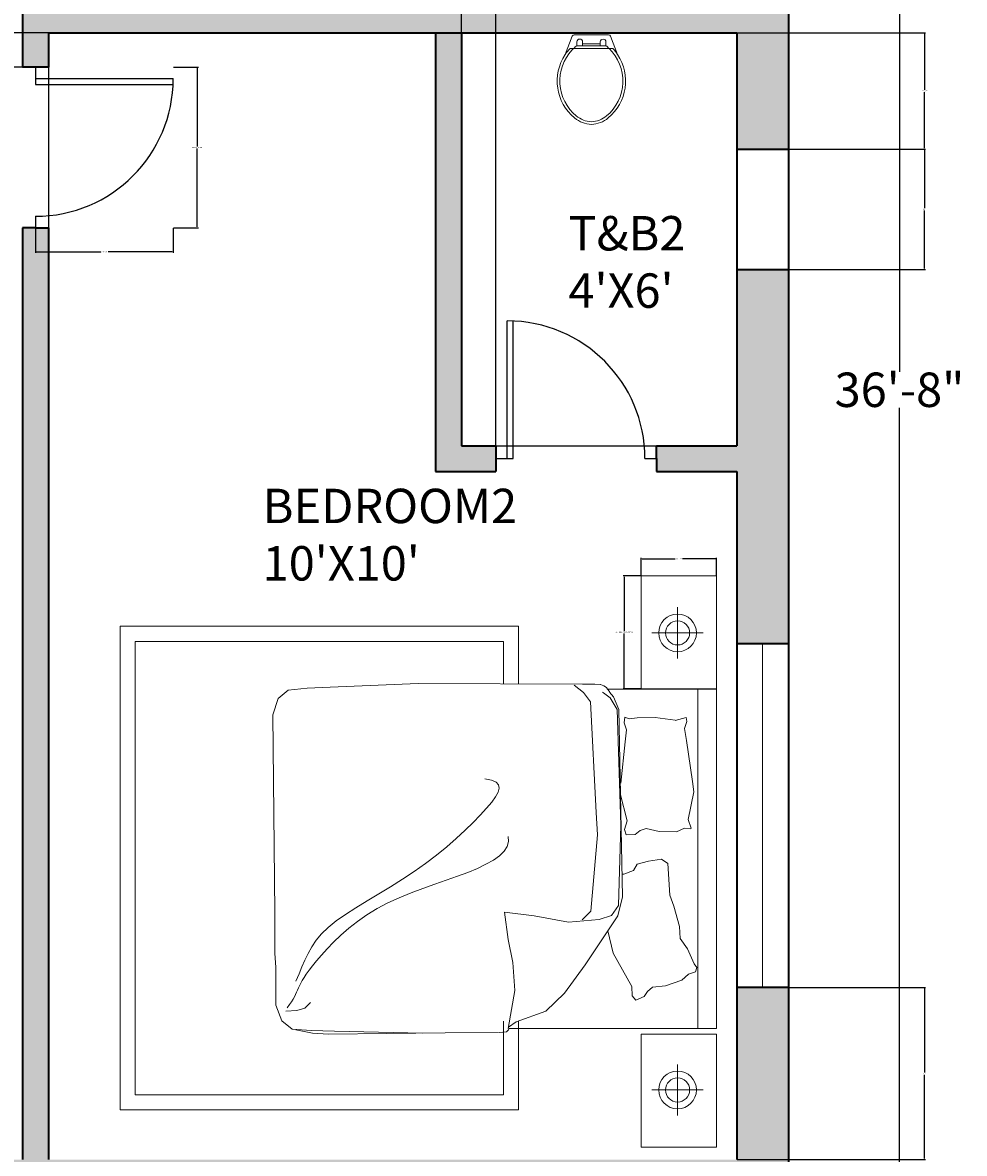
# Model space of a CAD drawing. Units: inches. Extents: x 10 to 332, y -471 to 73.
# Tile 3 of 5: x 168 to 332, y -341 to -144. Entities that reach past the tile are written whole.
import ezdxf

# ---------------------------------------------------------------- set-up
doc = ezdxf.new("R2010")
doc.units = ezdxf.units.IN
doc.header["$MEASUREMENT"] = 0
for name, color, linetype, lineweight in [('A-ANNO-DIMS', 2, 'Continuous', 18), ('A-AREA-IDEN', 7, 'Continuous', 18), ('A-DOOR', 3, 'Continuous', 25), ('A-FURN', 9, 'Continuous', 18), ('A-GLAZ', 4, 'Continuous', 18), ('A-WALL', 7, 'Continuous', 35), ('A-WALL-PATT', 8, 'Continuous', 13), ('WC-Detail_dwgmodels.com', 251, 'Continuous', 13), ('WC-Outline_dwgmodels.com', 250, 'Continuous', 18)]:
    doc.layers.add(name, color=color, linetype=linetype, lineweight=lineweight)
doc.styles.get("Standard").update_dxf_attribs({"font": 'arial.ttf'})
doc.dimstyles.get("Standard").update_dxf_attribs({"dimtxt": 0.18, "dimasz": 0.18, "dimexe": 0.18, "dimexo": 0.0625, "dimgap": 0.09, "dimtad": 0, "dimtih": 1, "dimtoh": 1, "dimdec": 0, "dimzin": 0, "dimdsep": 46, "dimlunit": 3, "dimtxsty": 'Standard', "dimcen": 0.09, "dimadec": 0, "dimazin": 0, "dimtfac": 1, "dimtdec": 0, "dimtofl": 0, "dimtmove": 0, "dimatfit": 3, "dimfxl": 1, "dimtolj": 1, "dimtzin": 0, "dimarcsym": 0})

# ---------------------------------------------------------------- blocks, each defined once
blk = doc.blocks.new('*D3')
at = {"layer": 'A-ANNO-DIMS', "color": 0, "lineweight": -2, "transparency": 16777216}
for p, q in [((301.43, 11.99), (320.92, 11.99)), ((320.74, 11.81), (320.74, -204.61)), ((320.74, -427.33), (320.74, -210.92)), ((301.43, -427.51), (320.92, -427.51))]:
    blk.add_line(p, q, dxfattribs=at)
at = {"layer": 'A-ANNO-DIMS', "color": 0, "transparency": 16777216}
for points in [[(320.71, 11.81), (320.77, 11.81), (320.74, 11.99)], [(320.71, -427.33), (320.77, -427.33), (320.74, -427.51)]]:
    blk.add_solid(points, dxfattribs=at)
at = {"layer": 'Defpoints', "color": 0, "transparency": 16777216}
for p in [(301.37, 11.99), (301.37, -427.51), (320.74, -427.51)]:
    blk.add_point(p, dxfattribs=at)
at = {"layer": 'A-ANNO-DIMS', "color": 0, "transparency": 16777216, "insert": (320.74, -207.76), "char_height": 6, "attachment_point": 5}
blk.add_mtext('\\A1;36\'-8"', dxfattribs=at)
blk = doc.blocks.new('DOOR-SINGLE-24')
for p, q in [((21.75, 0), (21.75, 28)), ((24, 26), (24, 28)), ((24, 3), (0, 3)), ((24, 2), (0, 2)), ((24, 2), (24, 3)), ((24, 0), (24, 2))]:
    blk.add_line(p, q)
blk.add_arc((24, 2), 24, 90, 180)
blk = doc.blocks.new('WIN-60')
for p, q in [((0, 9), (60, 9)), ((0, 4.5), (60, 4.5)), ((60, 0), (0, 0))]:
    blk.add_line(p, q)
blk = doc.blocks.new('NIGHTSTAND-20')
for p, q in [((6.34, 14.22), (6.34, 5.28)), ((10.81, 9.75), (1.87, 9.75))]:
    blk.add_line(p, q)
blk.add_lwpolyline([(0, 19.71), (0, 0), (13.14, 0), (13.14, 19.71)], close=True)
for radius in [3.29, 2.1]:
    blk.add_circle((6.34, 9.75), radius)
blk = doc.blocks.new('*D16')
at = {"layer": 'A-ANNO-DIMS', "color": 0, "lineweight": -2, "transparency": 16777216}
for p, q in [((194.18, -151.51), (198.5, -151.51)), ((198.32, -151.69), (198.32, -165.33)), ((198.32, -179.33), (198.32, -165.7)), ((194.18, -179.51), (198.5, -179.51))]:
    blk.add_line(p, q, dxfattribs=at)
at = {"layer": 'A-ANNO-DIMS', "color": 0, "transparency": 16777216}
for points in [[(198.29, -151.69), (198.35, -151.69), (198.32, -151.51)], [(198.29, -179.33), (198.35, -179.33), (198.32, -179.51)]]:
    blk.add_solid(points, dxfattribs=at)
at = {"layer": 'Defpoints', "color": 0, "transparency": 16777216}
for p in [(194.12, -151.51), (194.12, -179.51), (198.32, -179.51)]:
    blk.add_point(p, dxfattribs=at)
at = {"layer": 'A-ANNO-DIMS', "color": 0, "transparency": 16777216, "insert": (198.32, -165.51), "char_height": 0.18, "attachment_point": 5}
blk.add_mtext('\\A1;DOOR 2\'-4" TYP.', dxfattribs=at)
blk = doc.blocks.new('*D17')
at = {"layer": 'A-ANNO-DIMS', "color": 0, "lineweight": -2, "transparency": 16777216}
for p, q in [((170.12, -179.58), (170.12, -183.89)), ((194.12, -179.58), (194.12, -183.89)), ((170.3, -183.71), (181.48, -183.71)), ((193.94, -183.71), (182.76, -183.71))]:
    blk.add_line(p, q, dxfattribs=at)
at = {"layer": 'A-ANNO-DIMS', "color": 0, "transparency": 16777216}
for points in [[(170.3, -183.68), (170.3, -183.74), (170.12, -183.71)], [(193.94, -183.68), (193.94, -183.74), (194.12, -183.71)]]:
    blk.add_solid(points, dxfattribs=at)
at = {"layer": 'Defpoints', "color": 0, "transparency": 16777216}
for p in [(170.12, -179.51), (194.12, -179.51), (170.12, -183.71)]:
    blk.add_point(p, dxfattribs=at)
at = {"layer": 'A-ANNO-DIMS', "color": 0, "transparency": 16777216, "insert": (182.12, -183.71), "char_height": 0.18, "attachment_point": 5}
blk.add_mtext('\\A1;2\'-0" TYP.', dxfattribs=at)
blk = doc.blocks.new('*D22')
at = {"layer": 'A-ANNO-DIMS', "color": 0, "lineweight": -2, "transparency": 16777216}
for p, q in [((275.65, -240.21), (272.58, -240.21)), ((272.76, -240.39), (272.76, -249.88)), ((272.76, -259.73), (272.76, -250.24)), ((275.65, -259.91), (272.58, -259.91))]:
    blk.add_line(p, q, dxfattribs=at)
at = {"layer": 'A-ANNO-DIMS', "color": 0, "transparency": 16777216}
for points in [[(272.73, -240.39), (272.79, -240.39), (272.76, -240.21)], [(272.73, -259.73), (272.79, -259.73), (272.76, -259.91)]]:
    blk.add_solid(points, dxfattribs=at)
at = {"layer": 'Defpoints', "color": 0, "transparency": 16777216}
for p in [(272.76, -240.21), (275.71, -240.21), (275.71, -259.91)]:
    blk.add_point(p, dxfattribs=at)
at = {"layer": 'A-ANNO-DIMS', "color": 0, "transparency": 16777216, "insert": (272.76, -250.06), "char_height": 0.18, "attachment_point": 5}
blk.add_mtext('\\A1;NIGHTSTAND 1\'-7 1/2" TYP.', dxfattribs=at)
blk = doc.blocks.new('*D23')
at = {"layer": 'A-ANNO-DIMS', "color": 0, "lineweight": -2, "transparency": 16777216}
for p, q in [((275.71, -240.14), (275.71, -237.07)), ((275.89, -237.25), (281.65, -237.25)), ((288.67, -237.25), (282.91, -237.25)), ((288.85, -240.14), (288.85, -237.07))]:
    blk.add_line(p, q, dxfattribs=at)
at = {"layer": 'A-ANNO-DIMS', "color": 0, "transparency": 16777216}
for points in [[(275.89, -237.22), (275.89, -237.28), (275.71, -237.25)], [(288.67, -237.22), (288.67, -237.28), (288.85, -237.25)]]:
    blk.add_solid(points, dxfattribs=at)
at = {"layer": 'Defpoints', "color": 0, "transparency": 16777216}
for p in [(288.85, -237.25), (275.71, -240.21), (288.85, -240.21)]:
    blk.add_point(p, dxfattribs=at)
at = {"layer": 'A-ANNO-DIMS', "color": 0, "transparency": 16777216, "insert": (282.28, -237.25), "char_height": 0.18, "attachment_point": 5}
blk.add_mtext('\\A1;1\'-1" TYP.', dxfattribs=at)
blk = doc.blocks.new('*D42')
at = {"layer": 'A-ANNO-DIMS', "color": 0, "lineweight": -2, "transparency": 16777216}
for p, q in [((292.43, -145.51), (325.3, -145.51)), ((325.12, -145.69), (325.12, -155.47)), ((325.12, -165.61), (325.12, -155.84)), ((292.43, -165.79), (325.3, -165.79))]:
    blk.add_line(p, q, dxfattribs=at)
at = {"layer": 'A-ANNO-DIMS', "color": 0, "transparency": 16777216}
for points in [[(325.09, -145.69), (325.15, -145.69), (325.12, -145.51)], [(325.09, -165.61), (325.15, -165.61), (325.12, -165.79)]]:
    blk.add_solid(points, dxfattribs=at)
at = {"layer": 'Defpoints', "color": 0, "transparency": 16777216}
for p in [(292.37, -145.51), (292.37, -165.79), (325.12, -165.79)]:
    blk.add_point(p, dxfattribs=at)
at = {"layer": 'A-ANNO-DIMS', "color": 0, "transparency": 16777216, "insert": (325.12, -155.65), "char_height": 0.18, "attachment_point": 5}
blk.add_mtext('\\A1;1\'-8 1/2"', dxfattribs=at)
blk = doc.blocks.new('*D43')
at = {"layer": 'A-ANNO-DIMS', "color": 0, "lineweight": -2, "transparency": 16777216}
for p, q in [((301.43, -165.79), (325.3, -165.79)), ((325.12, -165.97), (325.12, -176.12)), ((325.12, -186.63), (325.12, -176.48)), ((301.43, -186.81), (325.3, -186.81))]:
    blk.add_line(p, q, dxfattribs=at)
at = {"layer": 'A-ANNO-DIMS', "color": 0, "transparency": 16777216}
for points in [[(325.09, -165.97), (325.15, -165.97), (325.12, -165.79)], [(325.09, -186.63), (325.15, -186.63), (325.12, -186.81)]]:
    blk.add_solid(points, dxfattribs=at)
at = {"layer": 'Defpoints', "color": 0, "transparency": 16777216}
for p in [(301.37, -165.79), (301.37, -186.81), (325.12, -186.81)]:
    blk.add_point(p, dxfattribs=at)
at = {"layer": 'A-ANNO-DIMS', "color": 0, "transparency": 16777216, "insert": (325.12, -176.3), "char_height": 0.18, "attachment_point": 5}
blk.add_mtext('\\A1;1\'-9"', dxfattribs=at)
blk = doc.blocks.new('*D44')
at = {"layer": 'A-ANNO-DIMS', "color": 0, "lineweight": -2, "transparency": 16777216}
for p, q in [((292.43, -312.01), (325.3, -312.01)), ((325.12, -312.19), (325.12, -326.83)), ((325.12, -341.83), (325.12, -327.2)), ((292.43, -342.01), (325.3, -342.01))]:
    blk.add_line(p, q, dxfattribs=at)
at = {"layer": 'A-ANNO-DIMS', "color": 0, "transparency": 16777216}
for points in [[(325.09, -312.19), (325.15, -312.19), (325.12, -312.01)], [(325.09, -341.83), (325.15, -341.83), (325.12, -342.01)]]:
    blk.add_solid(points, dxfattribs=at)
at = {"layer": 'Defpoints', "color": 0, "transparency": 16777216}
for p in [(292.37, -312.01), (292.37, -342.01), (325.12, -342.01)]:
    blk.add_point(p, dxfattribs=at)
at = {"layer": 'A-ANNO-DIMS', "color": 0, "transparency": 16777216, "insert": (325.12, -327.01), "char_height": 0.18, "attachment_point": 5}
blk.add_mtext('\\A1;2\'-6"', dxfattribs=at)
blk = doc.blocks.new('*D58')
at = {"layer": 'A-ANNO-DIMS', "color": 0, "lineweight": -2, "transparency": 16777216}
for p, q in [((172.3, -145.51), (10.44, -145.51)), ((10.62, -145.69), (10.62, -148.33)), ((10.62, -151.33), (10.62, -148.7)), ((167.8, -151.51), (10.44, -151.51))]:
    blk.add_line(p, q, dxfattribs=at)
at = {"layer": 'A-ANNO-DIMS', "color": 0, "transparency": 16777216}
for points in [[(10.59, -145.69), (10.65, -145.69), (10.62, -145.51)], [(10.59, -151.33), (10.65, -151.33), (10.62, -151.51)]]:
    blk.add_solid(points, dxfattribs=at)
at = {"layer": 'Defpoints', "color": 0, "transparency": 16777216}
for p in [(172.37, -145.51), (10.62, -151.51), (167.87, -151.51)]:
    blk.add_point(p, dxfattribs=at)
at = {"layer": 'A-ANNO-DIMS', "color": 0, "transparency": 16777216, "insert": (10.62, -148.51), "char_height": 0.18, "attachment_point": 5}
blk.add_mtext('\\A1;0\'-6"', dxfattribs=at)
blk = doc.blocks.new('*D59')
at = {"layer": 'A-ANNO-DIMS', "color": 0, "lineweight": -2, "transparency": 16777216}
for p, q in [((244.37, -217.45), (244.37, 35.92)), ((244.55, 35.74), (247.04, 35.74)), ((250.19, 35.74), (247.7, 35.74)), ((250.37, -217.45), (250.37, 35.92))]:
    blk.add_line(p, q, dxfattribs=at)
at = {"layer": 'A-ANNO-DIMS', "color": 0, "transparency": 16777216}
for points in [[(244.55, 35.77), (244.55, 35.71), (244.37, 35.74)], [(250.19, 35.77), (250.19, 35.71), (250.37, 35.74)]]:
    blk.add_solid(points, dxfattribs=at)
at = {"layer": 'Defpoints', "color": 0, "transparency": 16777216}
for p in [(250.37, 35.74), (244.37, -217.51), (250.37, -217.51)]:
    blk.add_point(p, dxfattribs=at)
at = {"layer": 'A-ANNO-DIMS', "color": 0, "transparency": 16777216, "insert": (247.37, 35.74), "char_height": 0.18, "attachment_point": 5}
blk.add_mtext('\\A1;0\'-6"', dxfattribs=at)

msp = doc.modelspace()

# ---------------------------------------------------------------- hatches: boundary and pattern name
at = {"layer": 'A-WALL-PATT'}
h = msp.add_hatch(color=256, dxfattribs=at)
h.dxf.hatch_style = 1
h.paths.add_polyline_path([(132.66, 11.99), (109.37, 11.99), (109.37, 2.99), (115.37, 2.99), (115.37, -93.01), (110.16, -93.01), (110.16, -97.51), (119.87, -97.51), (119.87, -73.51), (167.87, -73.51), (167.87, -107.01), (170.12, -107.01), (172.37, -107.01), (172.37, -63.01), (167.87, -63.01), (167.87, -69.01), (119.87, -69.01), (119.87, 2.99), (132.66, 2.99)])
h.paths.add_polyline_path([(202.37, 11.99), (152.96, 11.99), (152.96, 2.99), (167.87, 2.99), (167.87, -35.01), (170.12, -35.01), (172.37, -35.01), (172.37, 2.99), (202.37, 2.99)])
h.paths.add_polyline_path([(49.37, 11.99), (34.37, 11.99), (34.37, -15.01), (43.37, -15.01), (43.37, 2.99), (49.37, 2.99)])
h.paths.add_polyline_path([(301.37, 11.99), (262.37, 11.99), (262.37, 2.99), (292.37, 2.99), (292.37, -39.01), (301.37, -39.01)])
h.paths.add_polyline_path([(85.3, -93.01), (43.37, -93.01), (43.37, -75.01), (34.37, -75.01), (34.37, -165.2), (43.37, -165.2), (43.37, -97.51), (85.3, -97.51)])
h.paths.add_polyline_path([(43.37, -225.2), (34.37, -225.2), (34.37, -427.51), (49.37, -427.51), (49.37, -418.51), (43.37, -418.51), (43.37, -346.51), (49.4, -346.51), (49.4, -342.01), (43.37, -342.01)])
h.paths.add_polyline_path([(105.62, -342.01), (86.21, -342.01), (86.21, -346.51), (91.37, -346.51), (91.37, -418.51), (85.37, -418.51), (85.37, -427.51), (101.87, -427.51), (101.87, -418.51), (95.87, -418.51), (95.87, -346.51), (105.62, -346.51)])
h.paths.add_polyline_path([(301.37, -312.01), (292.37, -312.01), (292.37, -342.01), (172.37, -342.01), (172.37, -179.51), (170.12, -179.51), (167.87, -179.51), (167.87, -342.01), (158.84, -342.01), (158.84, -346.51), (292.37, -346.51), (292.37, -352.51), (301.37, -352.51)])
h.paths.add_polyline_path([(301.37, -412.51), (292.37, -412.51), (292.37, -418.51), (153.87, -418.51), (153.87, -423.01), (153.87, -427.51), (301.37, -427.51)])
h.paths.add_polyline_path([(301.37, -99.01), (292.37, -99.01), (292.37, -141.01), (172.37, -141.01), (172.37, -135.01), (167.87, -135.01), (167.87, -151.51), (172.37, -151.51), (172.37, -145.51), (292.37, -145.51), (292.37, -165.79), (301.37, -165.79)])
h = msp.add_hatch(color=256, dxfattribs=at)
h.dxf.hatch_style = 1
h.paths.add_polyline_path([(244.37, -145.51), (239.87, -145.51), (239.87, -222.01), (250.37, -222.01), (250.37, -217.51), (244.37, -217.51)])
h.paths.add_polyline_path([(301.37, -186.81), (292.37, -186.81), (292.37, -217.51), (278.37, -217.51), (278.37, -219.76), (278.37, -222.01), (292.37, -222.01), (292.37, -252.01), (301.37, -252.01)])

# ---------------------------------------------------------------- linework, layer by layer
at = {"layer": 'A-FURN'}
for p, q in [((214.18, -260.17), (212.43, -261.62)), ((217.49, -259.81), (214.18, -260.17)), ((221.5, -259.6), (217.49, -259.81)), ((236.85, -258.98), (221.5, -259.6)), ((265.48, -259.1), (236.85, -258.98)), ((267.62, -259.07), (265.48, -259.1)), ((268.54, -259.15), (267.62, -259.07)), ((269.84, -259.99), (288.85, -259.99)), ((212.43, -261.62), (211.48, -264.42)), ((211.86, -298.93), (211.48, -264.42)), ((281.62, -265.43), (283.53, -264.92)), ((283.87, -282.7), (284.87, -277.86)), ((284.87, -277.86), (284.68, -276.07)), ((273.26, -282.94), (272.03, -278.14)), ((272.78, -284.46), (273.26, -282.94)), ((284.41, -284.2), (283.87, -282.7)), ((273.08, -285.38), (272.78, -284.46)), ((274.66, -285.29), (273.08, -285.38)), ((275.51, -284.63), (274.66, -285.29)), ((276.58, -284.25), (275.51, -284.63)), ((278.82, -284.79), (276.58, -284.25)), ((281.84, -284.82), (278.82, -284.79)), ((283.27, -284.22), (281.84, -284.82)), ((284.37, -284.34), (283.27, -284.22)), ((284.37, -284.34), (283.27, -284.22)), ((284.37, -284.34), (284.41, -284.2)), ((280.36, -290.36), (280.69, -295.91)), ((280.69, -295.91), (281.4, -297.79)), ((211.86, -298.93), (211.86, -305.98)), ((281.4, -297.79), (282.36, -301.34)), ((282.36, -301.34), (282.53, -303.43)), ((282.53, -303.43), (283.76, -305.27)), ((282.53, -303.43), (283.76, -305.27)), ((283.76, -305.27), (284.97, -307.88)), ((211.86, -305.98), (212.04, -308.48)), ((274.09, -311.83), (270.82, -306)), ((212.04, -308.48), (212.04, -315.06)), ((282.81, -310.69), (279.96, -311.69)), ((283.95, -309.65), (282.81, -310.69)), ((274.15, -313.42), (274.09, -311.83)), ((274.75, -314.19), (274.15, -313.42)), ((276.79, -312.66), (276.21, -313.56)), ((277.67, -311.94), (276.79, -312.66)), ((279.96, -311.69), (277.67, -311.94)), ((213.07, -317.83), (212.04, -315.06)), ((217.05, -315.59), (218.06, -314.63)), ((276.21, -313.56), (274.75, -314.19)), ((213.75, -316.12), (215.7, -316.03)), ((215.7, -316.03), (217.05, -315.59)), ((214.87, -319.23), (213.07, -317.83)), ((218.18, -319.49), (214.87, -319.23)), ((215.47, -319.4), (218.4, -319.95)), ((252.57, -319.03), (252.62, -319.15)), ((222.21, -319.58), (218.18, -319.49)), ((218.4, -319.95), (221.22, -320.12)), ((221.22, -320.12), (241.56, -319.91)), ((237.57, -319.98), (222.21, -319.58)), ((241.56, -319.91), (250.84, -319.82))]:
    msp.add_line(p, q, dxfattribs=at)
for points in [[(254.3, -317.86), (254.3, -333.32), (184.86, -333.32), (184.86, -249), (254.3, -249), (254.3, -259.05)], [(251.68, -317.86), (251.68, -330.7), (187.49, -330.7), (187.49, -251.63), (251.68, -251.63), (251.68, -259.05)], [(288.85, -259.99), (288.85, -319.13), (252.67, -319.13)], [(265.43, -300.18), (266.94, -298.7), (268.08, -285.36), (267.85, -281.47), (266.88, -262.16), (265.65, -260.53), (264.01, -259.3)], [(268.6, -259.18), (269.21, -259.37), (269.68, -259.65), (269.84, -259.99), (270.18, -260.37), (270.2, -260.43)], [(285.57, -319.13), (285.57, -259.99)], [(252.54, -319.13), (253.7, -312.5), (253.33, -307.61), (252.52, -303.61), (251.86, -298.87), (257.03, -299.51), (263.05, -300.58), (268.37, -300.11), (270.52, -299.42), (271.75, -297.68), (272.13, -283.67), (271.53, -263.52), (270.31, -261.46), (269.11, -260.58), (268.99, -260.47)], [(270.19, -260.49), (270.9, -261.3), (271.83, -263.51), (272.47, -296.19), (271.63, -299.47), (268.14, -304.71), (265.96, -308.01), (262.32, -312.97), (259.1, -316.13), (253.93, -317.99), (252.58, -318.91)], [(272.15, -276.35), (272.9, -269.15), (273.16, -267.06), (272.71, -265.85), (272.84, -264.84), (273.63, -265.12), (275, -264.95), (278.16, -264.91), (281.62, -265.36)], [(284.68, -276.07), (283.6, -268.91), (283.25, -266.84), (283.65, -265.61), (283.53, -264.92)], [(215.51, -310.87), (216.06, -309.61), (216.57, -308.39), (217.07, -307.2), (217.62, -306.04), (218.26, -304.89), (219.03, -303.76), (219.97, -302.63), (221.13, -301.51), (222.54, -300.38), (224.17, -299.24), (225.97, -298.08), (227.91, -296.9), (229.94, -295.68), (232.02, -294.42), (234.1, -293.12), (236.15, -291.76), (238.13, -290.35), (240.02, -288.9), (241.81, -287.44), (243.47, -285.99), (245.01, -284.57), (246.41, -283.2), (247.66, -281.92), (248.74, -280.73), (249.64, -279.67), (250.32, -278.74), (250.78, -277.92), (250.96, -277.22), (250.85, -276.65), (250.41, -276.18), (249.62, -275.83), (248.44, -275.59)], [(213.96, -315.53), (214.38, -314.98), (214.72, -314.49), (215.01, -314.03), (215.24, -313.61), (215.45, -313.22), (215.62, -312.83), (215.79, -312.46), (215.96, -312.07), (216.14, -311.68), (216.35, -311.25), (216.61, -310.78), (216.93, -310.26), (217.32, -309.67), (217.8, -308.99), (218.39, -308.22), (219.11, -307.34), (219.96, -306.34), (220.94, -305.25), (222.06, -304.09), (223.32, -302.89), (224.71, -301.67), (226.22, -300.48), (227.87, -299.32), (229.65, -298.24), (231.55, -297.25), (233.54, -296.34), (235.58, -295.51), (237.65, -294.73), (239.71, -294), (241.73, -293.29), (243.66, -292.6), (245.48, -291.91), (247.15, -291.22), (248.65, -290.5), (249.94, -289.77), (251.01, -289.01), (251.82, -288.22), (252.36, -287.4), (252.59, -286.55), (252.49, -285.65)], [(280.36, -290.36), (279.27, -289.59), (276.99, -289.96), (274.98, -290.51), (274.34, -291.6), (272.7, -292.24), (272.39, -292.25)], [(270.82, -306), (269.87, -302.12)], [(283.95, -309.65), (285.16, -309.27), (285.41, -308.49), (284.97, -307.88)], [(250.93, -319.81), (252.21, -319.72), (252.59, -319.35), (252.67, -319.13)]]:
    msp.add_lwpolyline(points, dxfattribs=at)
at = {"layer": 'A-WALL'}
for p, q in [((301.37, 11.99), (301.37, -427.51)), ((167.87, -135.01), (167.87, -151.51)), ((172.37, -145.51), (292.37, -145.51)), ((172.37, -145.51), (172.37, -151.51)), ((239.87, -145.51), (239.87, -222.01)), ((244.37, -145.51), (244.37, -217.51)), ((292.37, -145.51), (292.37, -217.51)), ((172.37, -151.51), (167.87, -151.51)), ((292.37, -165.79), (301.37, -165.79)), ((170.12, -179.51), (167.87, -179.51)), ((167.87, -179.51), (167.87, -342.01)), ((170.12, -179.51), (172.37, -179.51)), ((172.37, -179.51), (172.37, -342.01)), ((292.37, -186.81), (301.37, -186.81)), ((244.37, -217.51), (250.37, -217.51)), ((250.37, -217.51), (250.37, -222.01)), ((278.37, -219.76), (278.37, -217.51)), ((278.37, -217.51), (292.37, -217.51)), ((278.37, -219.76), (278.37, -222.01)), ((239.87, -222.01), (250.37, -222.01)), ((278.37, -222.01), (292.37, -222.01)), ((292.37, -222.01), (292.37, -342.01)), ((292.37, -252.01), (301.37, -252.01)), ((301.37, -312.01), (292.37, -312.01))]:
    msp.add_line(p, q, dxfattribs=at)
at = {"layer": 'WC-Detail_dwgmodels.com'}
for p, q in [((263.3, -148.23), (263.96, -148.23)), ((270.1, -148.23), (270.76, -148.23))]:
    msp.add_line(p, q, dxfattribs=at)
for points in [[(264.49, -147.76, 0.022712), (263.96, -148.23, 0.162618)], [(264.49, -147.76), (264.49, -147.11, -1), (265.49, -147.11), (265.49, -147.45)], [(267.03, -147.76), (264.49, -147.76, 0.022712)], [(267.03, -147.76), (269.56, -147.76, -0.476108)], [(269.56, -147.76), (269.56, -147.11, 1), (268.57, -147.11), (268.57, -147.45)], [(269.56, -147.76, -0.022712), (270.1, -148.23, -0.162618)], [(263.3, -148.23, 0.040937), (262.45, -149.31, 0.163732)], [(270.76, -148.23, -0.040937), (271.6, -149.31, -0.163732)]]:
    msp.add_lwpolyline(points, format="xyb", dxfattribs=at)
for points in [[(268.57, -147.45), (265.49, -147.45)], [(265.49, -147.45), (265.49, -147.76)], [(268.57, -147.45), (268.57, -147.76)]]:
    msp.add_lwpolyline(points, dxfattribs=at)
at = {"layer": 'WC-Outline_dwgmodels.com'}
for p in [(263.96, -148.23), (270.1, -148.23)]:
    msp.add_line(p, (267.03, -148.23), dxfattribs=at)
for points in [[(267.03, -145.87), (264.05, -145.87, 0.31031), (263.68, -146.12), (262.45, -149.31, 0.209071)], [(267.03, -145.87), (270.01, -145.87, -0.31031), (270.38, -146.12), (271.6, -149.31, -0.209071)], [(262.45, -149.31, 0.383919), (264.09, -160.37, 0.163732), (267.03, -161.49, 0.359733)], [(263.64, -148.55, 0.431639), (264.39, -160.01, 0.162618), (267.03, -161.02, 0.470877)], [(263.96, -148.23, 0.014165), (263.64, -148.55, 0.162618)], [(270.1, -148.23, -0.448546), (269.67, -160.01, -0.162618), (267.03, -161.02, -0.470877)], [(271.6, -149.31, -0.383919), (269.96, -160.37, -0.163732), (267.03, -161.49, -0.359733)]]:
    msp.add_lwpolyline(points, format="xyb", dxfattribs=at)

# ---------------------------------------------------------------- block references
at = {"layer": 'A-DOOR'}
for p, rotation in [((194.12, -151.51), 180), ((250.37, -195.76), 270.0000000000001)]:
    msp.add_blockref('DOOR-SINGLE-24', p, dxfattribs=dict(at, rotation=rotation))
at = {"layer": 'A-FURN'}
msp.add_blockref('NIGHTSTAND-20', (275.71, -259.91), dxfattribs=at)
at = {"layer": 'A-FURN', "extrusion": (0, 0, -1), "zscale": -1, "rotation": 180}
msp.add_blockref('NIGHTSTAND-20', (-275.71, -320.11), dxfattribs=at)
at = {"layer": 'A-GLAZ', "rotation": 270}
msp.add_blockref('WIN-60', (292.37, -252.01), dxfattribs=at)

# ---------------------------------------------------------------- texts
at = {"layer": 'A-AREA-IDEN', "char_height": 6, "attachment_point": 1}
for s, insert in [("T&B2\\P4'X6'", (263.03, -177.47)), ("BEDROOM2\\P10'X10'", (209.71, -225.02))]:
    msp.add_mtext(s, dxfattribs=dict(at, insert=insert))

# ---------------------------------------------------------------- dimensions: what is measured, and where the dimension line sits
at = {"layer": 'A-ANNO-DIMS'}
dim = msp.add_linear_dim(base=(250.37, 35.74), p1=(244.37, -217.51), p2=(250.37, -217.51), dimstyle='Standard', override={"dimdec": 1, "dimlfac": 1, "dimrnd": 0, "dimzin": 1, "dimdsep": 46, "dimlunit": 4, "dimfrac": 2}, dxfattribs=at)
dim.commit()
dim.dimension.update_dxf_attribs({"geometry": '*D59', "text_midpoint": (247.37, 35.74)})
for base, p1, p2, override, picture, middle in [((320.73862044, -427.51494379), (301.36648826, 11.98505621), (301.36648826, -427.51494379), {"dimtxt": 6, "dimclrd": 0, "dimclre": 0, "dimclrt": 0}, '*D3', (320.73862044, -207.76494379)), ((10.62, -151.51), (172.37, -145.51), (167.87, -151.51), {"dimdec": 1, "dimlfac": 1, "dimrnd": 0, "dimzin": 1, "dimdsep": 46, "dimlunit": 4, "dimfrac": 2}, '*D58', (10.62, -148.51)), ((325.12, -165.79), (292.37, -145.51), (292.37, -165.79), {"dimdec": 1, "dimlfac": 1, "dimrnd": 0, "dimzin": 1, "dimdsep": 46, "dimlunit": 4, "dimfrac": 2}, '*D42', (325.12, -155.65)), ((325.12, -186.81), (301.37, -165.79), (301.37, -186.81), {"dimdec": 1, "dimlfac": 1, "dimrnd": 0, "dimzin": 1, "dimdsep": 46, "dimlunit": 4, "dimfrac": 2}, '*D43', (325.12, -176.3)), ((325.12, -342.01), (292.37, -312.01), (292.37, -342.01), {"dimdec": 1, "dimlfac": 1, "dimrnd": 0, "dimzin": 1, "dimdsep": 46, "dimlunit": 4, "dimfrac": 2}, '*D44', (325.12, -327.01))]:
    dim = msp.add_linear_dim(base=base, p1=p1, p2=p2, angle=90, dimstyle='Standard', override=override, dxfattribs=at)
    dim.commit()
    dim.dimension.update_dxf_attribs({"geometry": picture, "text_midpoint": middle})
for base, p1, p2, angle, text, picture, middle in [((198.32, -179.51), (194.12, -151.51), (194.12, -179.51), 270, 'DOOR <> TYP.', '*D16', (198.32, -165.51)), ((170.12, -183.71), (194.12, -179.51), (170.12, -179.51), 180, '<> TYP.', '*D17', (182.12, -183.71)), ((272.76, -240.21), (275.71, -259.91), (275.71, -240.21), 90, 'NIGHTSTAND <> TYP.', '*D22', (272.76, -250.06))]:
    dim = msp.add_linear_dim(base=base, p1=p1, p2=p2, angle=angle, text=text, dimstyle='Standard', override={"dimdec": 1, "dimlfac": 1, "dimrnd": 0, "dimzin": 1, "dimdsep": 46, "dimlunit": 4, "dimfrac": 2}, dxfattribs=at)
    dim.commit()
    dim.dimension.update_dxf_attribs({"geometry": picture, "text_midpoint": middle})
dim = msp.add_linear_dim(base=(288.85, -237.25), p1=(275.71, -240.21), p2=(288.85, -240.21), text='<> TYP.', dimstyle='Standard', override={"dimdec": 1, "dimlfac": 1, "dimrnd": 0, "dimzin": 1, "dimdsep": 46, "dimlunit": 4, "dimfrac": 2}, dxfattribs=at)
dim.commit()
dim.dimension.update_dxf_attribs({"geometry": '*D23', "text_midpoint": (282.28, -237.25)})

doc.saveas('drawing.dxf')
